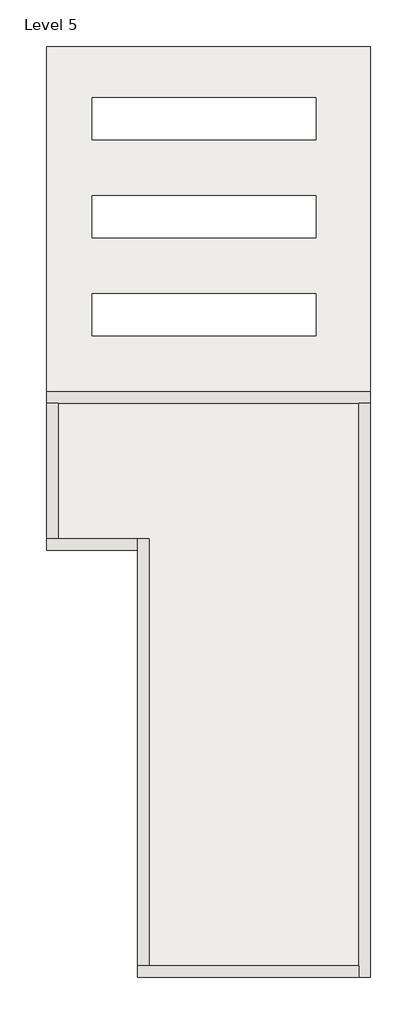
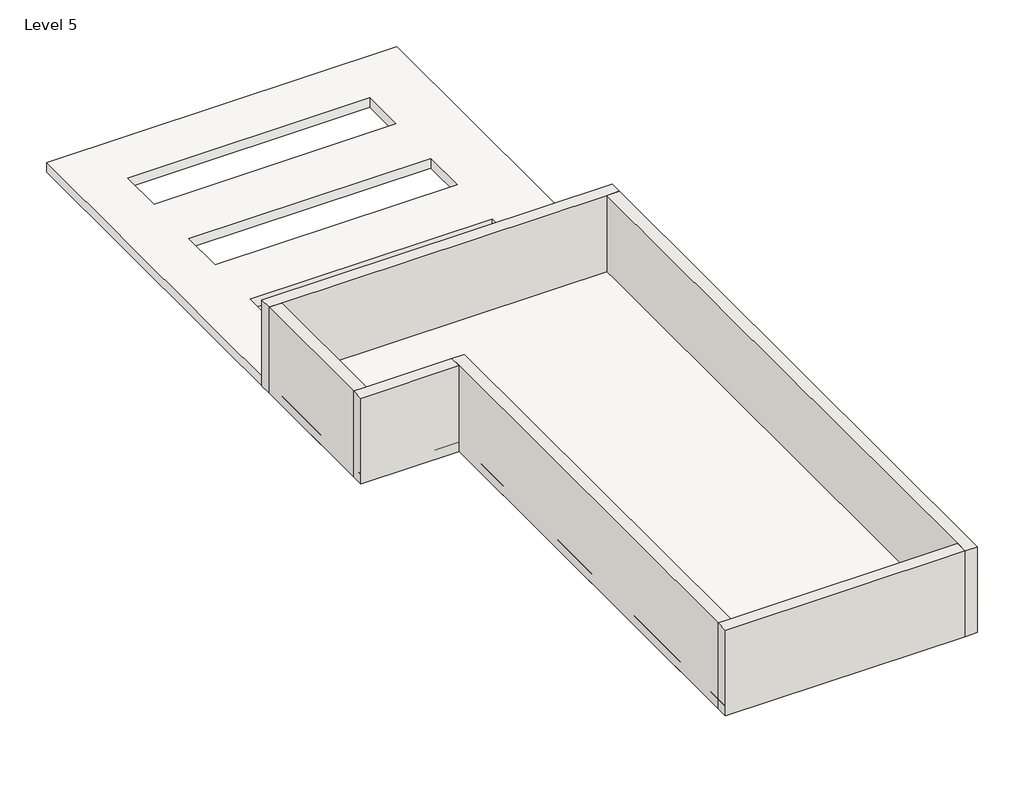
# One storey: 6 walls, 1 roof.
"""IFC4 building model written with IfcOpenShell, lengths in millimetres."""

from ifc_helpers import new_model, si_unit, frame, origin, place, context, project, spatial, polyline, outline, extrude, faceted_brep, element, save

model = new_model("IFC4")

# Units and contexts
model_context = context("Model", 3, world=origin())
ifc_project = project(units=[si_unit("LENGTHUNIT", "METRE", prefix="MILLI")], contexts=[model_context])

# Site, building, storey
site = spatial("IfcSite", under=ifc_project)
building = spatial("IfcBuilding", under=site)
storey = spatial("IfcBuildingStorey", under=building, Name="Level 5", Elevation=12192.0)

# Roof
placement = place(None, origin())
element("IfcRoof", 1, ObjectType="Generic - 4\"", at=placement, inside=storey, context=model_context, shape_type="SweptSolid", body=[
    extrude(outline(polyline([(-11332.3394758, 12774.4495492), (-7801.7394758, 12774.4495492), (-7801.7394758, 2639.8495492), (-10341.7394758, 2639.8495492), (-10341.7394758, 7288.0495492), (-11332.3394758, 7288.0495492), (-11332.3394758, 12774.4495492)]), holes=[polyline([(-8397.2079028, 11758.3218329), (-8397.2079028, 12215.5218329), (-10835.6079028, 12215.5218329), (-10835.6079028, 11758.3218329), (-8397.2079028, 11758.3218329)]), polyline([(-8397.2079028, 10691.5218329), (-8397.2079028, 11148.7218329), (-10835.6079028, 11148.7218329), (-10835.6079028, 10691.5218329), (-8397.2079028, 10691.5218329)]), polyline([(-8397.2079028, 9624.7218329), (-8397.2079028, 10081.9218329), (-10835.6079028, 10081.9218329), (-10835.6079028, 9624.7218329), (-8397.2079028, 9624.7218329)])]), frame((0.0, 0.0, 12192.0), z_axis=(0.0, 0.0, 1.0), x_axis=(1.0, 0.0, 0.0)), (0.0, 0.0, 1.0), 101.6),
])

# Walls
element("IfcWall", 2, ObjectType="Generic - 5\"", at=placement, inside=storey, context=model_context, shape_type="Brep", body=[
    faceted_brep([(-11332.3394758, 8888.2495492, 12192.0), (-11205.3394758, 8888.2495492, 12192.0), (-7928.7394758, 8888.2495492, 12192.0), (-7801.7394758, 8888.2495492, 12192.0), (-7801.7394758, 8888.2495492, 13106.4), (-7928.7394758, 8888.2495492, 13106.4), (-11205.3394758, 8888.2495492, 13106.4), (-11332.3394758, 8888.2495492, 13106.4), (-11332.3394758, 9015.2495492, 12192.0), (-11332.3394758, 9015.2495492, 13106.4), (-7801.7394758, 9015.2495492, 13106.4), (-7801.7394758, 9015.2495492, 12192.0)], [[[0, 1, 2, 3, 4, 5, 6, 7]], [[8, 9, 10, 11]], [[3, 2, 1, 0, 8, 11]], [[7, 6, 5, 4, 10, 9]], [[4, 3, 11, 10]], [[0, 7, 9, 8]]]),
])
element("IfcWall", 3, ObjectType="Generic - 5\"", at=placement, inside=storey, context=model_context, shape_type="Brep", body=[
    faceted_brep([(-7928.7394758, 8888.2495492, 12192.0), (-7928.7394758, 2766.8495492, 12192.0), (-7928.7394758, 2639.8495492, 12192.0), (-7928.7394758, 2639.8495492, 13106.4), (-7928.7394758, 2766.8495492, 13106.4), (-7928.7394758, 8888.2495492, 13106.4), (-7801.7394758, 8888.2495492, 12192.0), (-7801.7394758, 8888.2495492, 13106.4), (-7801.7394758, 2639.8495492, 13106.4), (-7801.7394758, 2639.8495492, 12192.0)], [[[0, 1, 2, 3, 4, 5]], [[6, 7, 8, 9]], [[2, 1, 0, 6, 9]], [[5, 4, 3, 8, 7]], [[0, 5, 7, 6]], [[3, 2, 9, 8]]]),
])
element("IfcWall", 4, ObjectType="Generic - 5\"", at=placement, inside=storey, context=model_context, shape_type="Brep", body=[
    faceted_brep([(-7928.7394758, 2766.8495492, 12192.0), (-10214.7394758, 2766.8495492, 12192.0), (-10341.7394758, 2766.8495492, 12192.0), (-10341.7394758, 2766.8495492, 13106.4), (-10214.7394758, 2766.8495492, 13106.4), (-7928.7394758, 2766.8495492, 13106.4), (-7928.7394758, 2639.8495492, 12192.0), (-7928.7394758, 2639.8495492, 13106.4), (-10341.7394758, 2639.8495492, 13106.4), (-10341.7394758, 2639.8495492, 12192.0)], [[[0, 1, 2, 3, 4, 5]], [[6, 7, 8, 9]], [[2, 1, 0, 6, 9]], [[5, 4, 3, 8, 7]], [[0, 5, 7, 6]], [[3, 2, 9, 8]]]),
])
element("IfcWall", 5, ObjectType="Generic - 5\"", at=placement, inside=storey, context=model_context, shape_type="Brep", body=[
    faceted_brep([(-10214.7394758, 2766.8495492, 12192.0), (-10214.7394758, 7415.0495492, 12192.0), (-10214.7394758, 7415.0495492, 13106.4), (-10214.7394758, 2766.8495492, 13106.4), (-10341.7394758, 2766.8495492, 12192.0), (-10341.7394758, 2766.8495492, 13106.4), (-10341.7394758, 7288.0495492, 13106.4), (-10341.7394758, 7415.0495492, 13106.4), (-10341.7394758, 7415.0495492, 12192.0), (-10341.7394758, 7288.0495492, 12192.0)], [[[0, 1, 2, 3]], [[4, 5, 6, 7, 8, 9]], [[1, 0, 4, 9, 8]], [[3, 2, 7, 6, 5]], [[0, 3, 5, 4]], [[2, 1, 8, 7]]]),
])
element("IfcWall", 6, ObjectType="Generic - 5\"", at=placement, inside=storey, context=model_context, shape_type="Brep", body=[
    faceted_brep([(-10341.7394758, 7415.0495492, 12192.0), (-11205.3394758, 7415.0495492, 12192.0), (-11332.3394758, 7415.0495492, 12192.0), (-11332.3394758, 7415.0495492, 13106.4), (-11205.3394758, 7415.0495492, 13106.4), (-10341.7394758, 7415.0495492, 13106.4), (-10341.7394758, 7288.0495492, 12192.0), (-10341.7394758, 7288.0495492, 13106.4), (-11332.3394758, 7288.0495492, 13106.4), (-11332.3394758, 7288.0495492, 12192.0)], [[[0, 1, 2, 3, 4, 5]], [[6, 7, 8, 9]], [[2, 1, 0, 6, 9]], [[5, 4, 3, 8, 7]], [[0, 5, 7, 6]], [[3, 2, 9, 8]]]),
])
element("IfcWall", 7, ObjectType="Generic - 5\"", at=placement, inside=storey, context=model_context, shape_type="SweptSolid", body=[
    extrude(outline(polyline([(-11205.3394758, 8888.2495492), (-11205.3394758, 7415.0495492), (-11332.3394758, 7415.0495492), (-11332.3394758, 8888.2495492), (-11205.3394758, 8888.2495492)])), frame((0.0, 0.0, 12192.0), z_axis=(0.0, 0.0, 1.0), x_axis=(1.0, 0.0, 0.0)), (0.0, 0.0, 1.0), 914.4),
])

save(model, "model.ifc")

# Revit data of these elements
# Type "Generic - 4\""
#   Assembly Code = "B1020"
#   Layers, outside or top first: 0' - 4" "01 colour 1" (function 1)
# Type "Generic - 5\""
#   Assembly Code = "B2010"
#   Layers, outside or top first: 0' - 5" no material (function 1)
# Element 1 (IfcRoof, "Generic - 4\"")
#   built-in parameter 1001705 = 40.3333 (stored number, unit not read)
#   built-in parameter 1001710 = 33615
#   Phase Created = New Construction
#   Materials on its faces: "01 colour 1"
# Elements 2, 3, 4, 5, 6, 7 (IfcWall, "Generic - 5\"")
#   Top Offset = 0' - 0"
#   Base Offset = 0' - 0"
#   Unconnected Height = 3' - 0"
#   wall height = 3' - 0"
#   Phase Created = New Construction
#   Base Constraint = Level 5
#   Materials on its faces: "Default Wall", "01 colour 1"
# Materials
#   "01 colour 1": class "Generic", colour RGB 120 120 120, transparency 0, Cost = 0
#   "Default Wall": colour RGB 80 80 80, transparency 0
